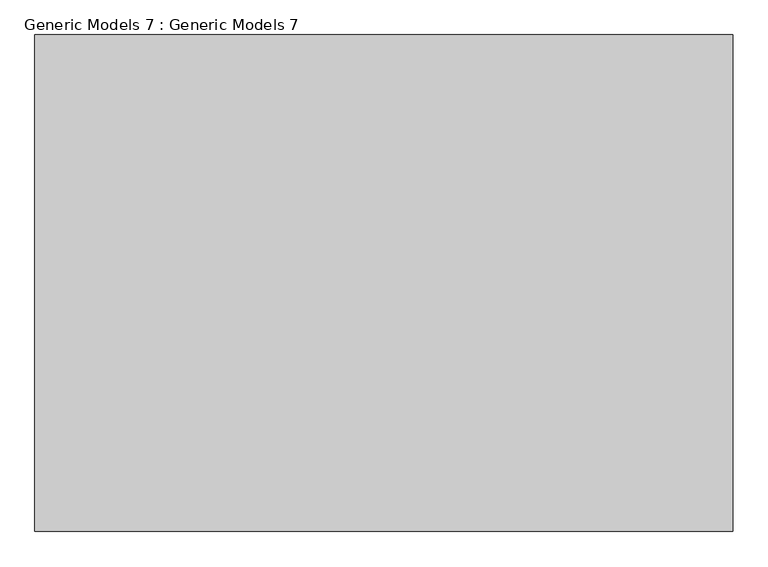
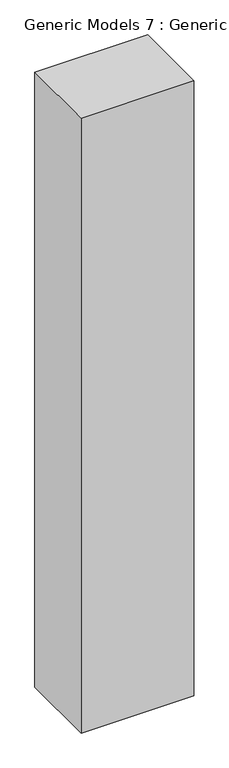
"""IFC4 building model written with IfcOpenShell, lengths in millimetres: proxy geometry, Generic Models 7 : Generic Models 7."""

from ifc_helpers import new_model, si_unit, origin, origin_with_axes, place, context, project, spatial, polyline, outline, extrude, source, transform, mapped, element, save


def generic_models_7_generic_models_7_5b8c9dda(model_context):
    return source(origin(), model_context, "Body", "SweptSolid", [
        extrude(outline(polyline([(1802.1364313, -8492.7980299), (1802.1364313, -9283.4202021), (691.2877114, -9283.4202021), (691.2877114, -8492.7980299), (1802.1364313, -8492.7980299)])), origin_with_axes(), (0.0, 0.0, 1.0), 6410.9930152),
    ])


if __name__ == "__main__":
    model = new_model("IFC4")
    model_context = context("Model", 3, world=origin())
    ifc_project = project(units=[si_unit("LENGTHUNIT", "METRE", prefix="MILLI")], contexts=[model_context])
    site = spatial("IfcSite", under=ifc_project)
    building = spatial("IfcBuilding", under=site)
    placement = place(None, origin())
    generic_models_7_generic_models_7_shape = generic_models_7_generic_models_7_5b8c9dda(model_context)
    element("IfcBuildingElementProxy", 1, Name="Generic Models 7 : Generic Models 7", ObjectType="Generic Models 7 : Generic Models 7", at=placement, inside=building, context=model_context, shape_type="MappedRepresentation", body=[
        mapped(generic_models_7_generic_models_7_shape, transform((0.0, 0.0, 0.0), x_axis=(1.0, 0.0, 0.0), y_axis=(0.0, 1.0, 0.0), z_axis=(0.0, 0.0, 1.0))),
    ])
    save(model, "model.ifc")
